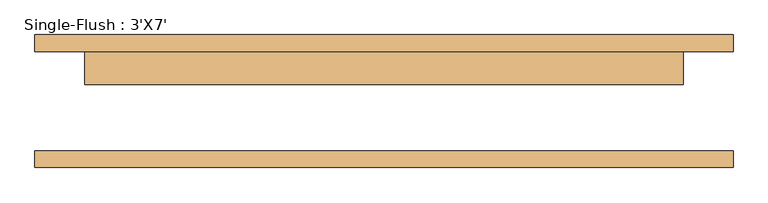
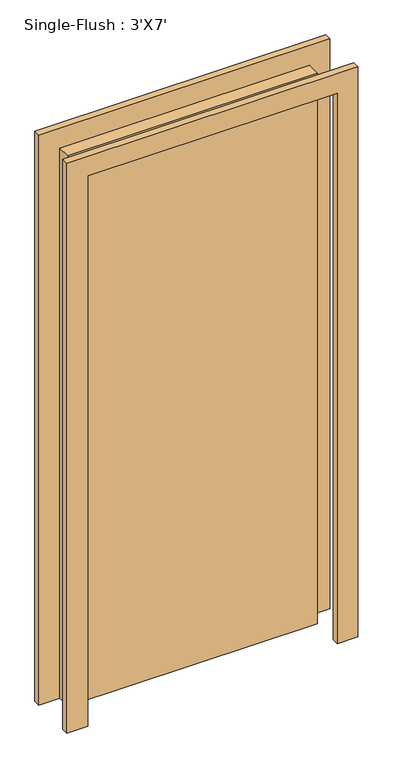
"""IFC4 building model written with IfcOpenShell, lengths in millimetres: door geometry, Single-Flush : 3'X7'."""

from ifc_helpers import new_model, si_unit, frame, origin, origin_with_axes, place, context, project, spatial, polyline, outline, extrude, source, transform, mapped, element, save


def single_flush_3_x7_16372e1c(model_context):
    return source(origin(), model_context, "Body", "SweptSolid", [
        extrude(outline(polyline([(2209.8, -533.4), (0.0, -533.4), (0.0, -457.2), (2133.6, -457.2), (2133.6, 457.2), (0.0, 457.2), (0.0, 533.4), (2209.8, 533.4), (2209.8, -533.4)])), frame((0.0, 76.2, 0.0), z_axis=(0.0, 1.0, 0.0), x_axis=(0.0, 0.0, 1.0)), (0.0, 0.0, 1.0), 25.4),
        extrude(outline(polyline([(2209.8, 533.4), (2209.8, -533.4), (0.0, -533.4), (0.0, -457.2), (2133.6, -457.2), (2133.6, 457.2), (0.0, 457.2), (0.0, 533.4), (2209.8, 533.4)])), frame((0.0, -101.6, 0.0), z_axis=(0.0, 1.0, 0.0), x_axis=(0.0, 0.0, 1.0)), (0.0, 0.0, 1.0), 25.4),
        extrude(outline(polyline([(457.2, 25.4), (-457.2, 25.4), (-457.2, 76.2), (457.2, 76.2), (457.2, 25.4)])), origin_with_axes(), (0.0, 0.0, 1.0), 2133.6),
    ])


if __name__ == "__main__":
    model = new_model("IFC4")
    model_context = context("Model", 3, world=origin())
    ifc_project = project(units=[si_unit("LENGTHUNIT", "METRE", prefix="MILLI")], contexts=[model_context])
    site = spatial("IfcSite", under=ifc_project)
    building = spatial("IfcBuilding", under=site)
    placement = place(None, origin())
    single_flush_3_x7_shape = single_flush_3_x7_16372e1c(model_context)
    element("IfcDoor", 1, ObjectType="Single-Flush : 3'X7'", at=placement, inside=building, context=model_context, shape_type="MappedRepresentation", body=[
        mapped(single_flush_3_x7_shape, transform((0.0, 0.0, 0.0), x_axis=(1.0, 0.0, 0.0), y_axis=(0.0, 1.0, 0.0), z_axis=(0.0, 0.0, 1.0))),
    ])
    save(model, "model.ifc")

# Revit data of these elements
# Type "Single-Flush : 3'X7'"
#   Type Mark = "8"
#   Construction Type Id = "MDOOR"
#   Assembly Code = "C1020"
#   Analytic Construction = "Metal"
#   Thickness = 0' - 2"
#   Heat Transfer Coefficient (U) = 0.651978 BTU/(h·ft²·°F)
#   Height = 7' - 0"
#   Trim Projection Ext = 0' - 1"
#   Trim Projection Int = 0' - 1"
#   Trim Width = 0' - 3"
#   Width = 3' - 0"
#   Define Thermal Properties by = 1
#   Door Material = Door - Panel
#   Frame Material = Door - Frame
#   Visual Light Transmittance = 0
#   Solar Heat Gain Coefficient = 0
#   Function = (empty or 0)
#   Wall Closure = (empty or 0)
# Element 1 (IfcDoor, "Single-Flush : 3'X7'")
#   Materials on its faces: "Door - Frame", "Door - Panel"
# Materials
#   "Door - Panel": class "Wood", colour RGB 210 159 95, transparency 0, Cost = 0
#   "Door - Frame": colour RGB 118 70 51, transparency 0, Cost = 0
